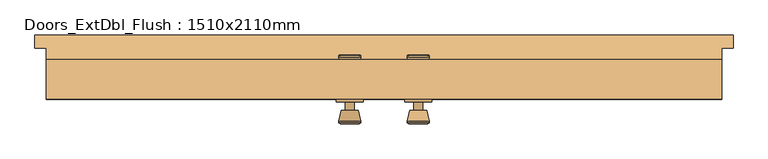
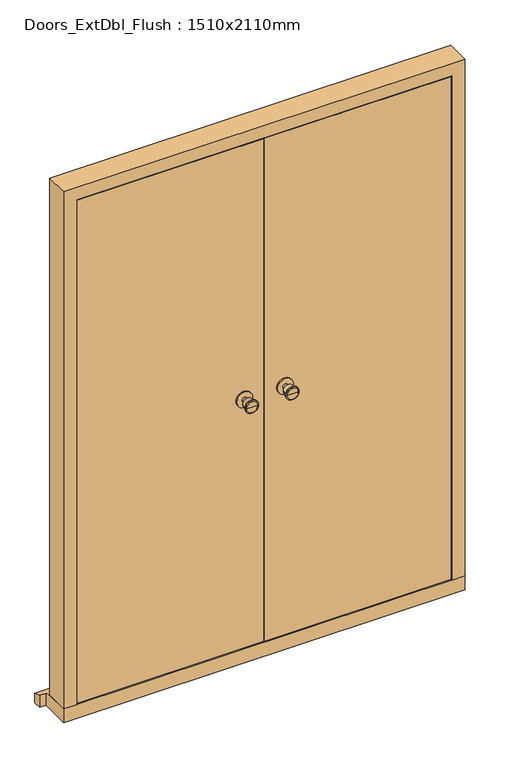
"""IFC4 building model written with IfcOpenShell, lengths in millimetres: door geometry, Doors_ExtDbl_Flush : 1510x2110mm."""

from ifc_helpers import new_model, si_unit, point, frame, frame_2d, origin, place, context, project, spatial, polyline, circle_curve, trimmed, segment, composite_curve, outline, extrude, faceted_brep, source, transform, mapped, element, save
from ifc_brep_helpers import plane_surface, cylinder_surface, revolved_surface, advanced_brep


def doors_extdbl_flush_1510x2110mm_6aadbff8(model_context):
    return source(origin(), model_context, "Body", "SolidModel", [
        advanced_brep(
        [(-76.5, -62.85, 1050.0), (-66.5, -62.85, 1050.0), (-86.5, -62.85, 1050.0), (-96.9758676, -111.85, 1050.0), (-56.0241324, -111.85, 1050.0), (-76.5, -111.85, 1050.0), (-101.5, -110.0221319, 1050.0), (-51.5, -110.0221319, 1050.0), (-101.5, -106.5584537, 1050.0), (-51.5, -106.5584537, 1050.0), (-95.136236, -81.85, 1050.0), (-57.863764, -81.85, 1050.0), (-86.5, -81.85, 1050.0), (-66.5, -81.85, 1050.0)],
        [
            (0, 1),
            (1, 2, circle_curve(frame((-76.5, -62.85, 1050.0), z_axis=(0.0, 1.0, 0.0), x_axis=(1.0, 0.0, 0.0)), 10.0)),
            (2, 0),
            (2, 1, circle_curve(frame((-76.5, -62.85, 1050.0), z_axis=(0.0, 1.0, 0.0), x_axis=(1.0, 0.0, 0.0)), 10.0)),
            (3, 4, circle_curve(frame((-76.5, -111.85, 1050.0), z_axis=(0.0, -1.0, 0.0), x_axis=(1.0, 0.0, 0.0)), 20.4758676)),
            (4, 5),
            (5, 3),
            (4, 3, circle_curve(frame((-76.5, -111.85, 1050.0), z_axis=(0.0, -1.0, 0.0), x_axis=(1.0, 0.0, 0.0)), 20.4758676)),
            (6, 7, circle_curve(frame((-76.5, -110.0221319, 1050.0), z_axis=(0.0, -1.0, 0.0), x_axis=(1.0, 0.0, 0.0)), 25.0)),
            (7, 4),
            (3, 6),
            (7, 6, circle_curve(frame((-76.5, -110.0221319, 1050.0), z_axis=(0.0, -1.0, 0.0), x_axis=(1.0, 0.0, 0.0)), 25.0)),
            (8, 9, circle_curve(frame((-76.5, -106.5584537, 1050.0), z_axis=(0.0, -1.0, 0.0), x_axis=(1.0, 0.0, 0.0)), 25.0)),
            (9, 7),
            (6, 8),
            (9, 8, circle_curve(frame((-76.5, -106.5584537, 1050.0), z_axis=(0.0, -1.0, 0.0), x_axis=(1.0, 0.0, 0.0)), 25.0)),
            (10, 11, circle_curve(frame((-76.5, -81.85, 1050.0), z_axis=(0.0, -1.0, 0.0), x_axis=(1.0, 0.0, 0.0)), 18.636236)),
            (11, 9),
            (8, 10),
            (11, 10, circle_curve(frame((-76.5, -81.85, 1050.0), z_axis=(0.0, -1.0, 0.0), x_axis=(1.0, 0.0, 0.0)), 18.636236)),
            (12, 13, circle_curve(frame((-76.5, -81.85, 1050.0), z_axis=(0.0, -1.0, 0.0), x_axis=(1.0, 0.0, 0.0)), 10.0)),
            (13, 11),
            (10, 12),
            (13, 12, circle_curve(frame((-76.5, -81.85, 1050.0), z_axis=(0.0, -1.0, 0.0), x_axis=(1.0, 0.0, 0.0)), 10.0)),
            (1, 13),
            (12, 2),
        ],
        [
            plane_surface(frame((-76.5, -62.85, 1050.0), z_axis=(0.0, 1.0, 0.0), x_axis=(1.0, 0.0, 0.0))),
            plane_surface(frame((-76.5, -111.85, 1050.0), z_axis=(0.0, -1.0, 0.0), x_axis=(1.0, 0.0, 0.0))),
            revolved_surface(polyline([(-56.0241324, -111.85, 1050.0), (-51.5, -110.0221319, 1050.0)]), (-76.5, -62.85, 1050.0), (0.0, 1.0, 0.0)),
            cylinder_surface(frame((-76.5, -62.85, 1050.0), z_axis=(0.0, 1.0, 0.0), x_axis=(1.0, 0.0, 0.0)), 25.0),
            revolved_surface(polyline([(-51.5, -106.5584537, 1050.0), (-57.863764, -81.85, 1050.0)]), (-76.5, -62.85, 1050.0), (0.0, 1.0, 0.0)),
            plane_surface(frame((-76.5, -81.85, 1050.0), z_axis=(0.0, 1.0, 0.0), x_axis=(1.0, 0.0, 0.0))),
            cylinder_surface(frame((-76.5, -62.85, 1050.0), z_axis=(0.0, 1.0, 0.0), x_axis=(1.0, 0.0, 0.0)), 10.0),
        ],
        [
            (0, [[1, 2, 3]]),
            (0, [[-3, 4, -1]]),
            (1, [[5, 6, 7]]),
            (1, [[8, -7, -6]]),
            (2, [[9, 10, -5, 11]]),
            (2, [[12, -11, -8, -10]]),
            (3, [[13, 14, -9, 15]]),
            (3, [[16, -15, -12, -14]]),
            (4, [[17, 18, -13, 19]]),
            (4, [[20, -19, -16, -18]]),
            (5, [[21, 22, -17, 23]]),
            (5, [[24, -23, -20, -22]]),
            (6, [[-2, 25, -21, 26]]),
            (6, [[-4, -26, -24, -25]]),
        ],
    ),
        extrude(outline(composite_curve([segment(trimmed(circle_curve(frame_2d((1050.0, -76.5)), 30.0), [point((1050.0, -46.5))], [point((1050.0, -106.5))], False, "CARTESIAN"), True, "CONTINUOUS"), segment(trimmed(circle_curve(frame_2d((1050.0, -76.5)), 30.0), [point((1050.0, -106.5))], [point((1050.0, -46.5))], False, "CARTESIAN"), True, "CONTINUOUS")], self_intersect=False)), frame((0.0, -62.85, 0.0), z_axis=(0.0, 1.0, 0.0), x_axis=(0.0, 0.0, 1.0)), (0.0, 0.0, 1.0), 6.0),
        advanced_brep(
        [(-76.5, -6.85, 1050.0), (-86.5, -6.85, 1050.0), (-66.5, -6.85, 1050.0), (-96.9758676, 42.15, 1050.0), (-76.5, 42.15, 1050.0), (-56.0241324, 42.15, 1050.0), (-101.5, 40.3221319, 1050.0), (-51.5, 40.3221319, 1050.0), (-101.5, 36.8584537, 1050.0), (-51.5, 36.8584537, 1050.0), (-95.136236, 12.15, 1050.0), (-57.863764, 12.15, 1050.0), (-86.5, 12.15, 1050.0), (-66.5, 12.15, 1050.0)],
        [
            (0, 1),
            (1, 2, circle_curve(frame((-76.5, -6.85, 1050.0), z_axis=(0.0, -1.0, 0.0), x_axis=(1.0, 0.0, 0.0)), 10.0)),
            (2, 0),
            (2, 1, circle_curve(frame((-76.5, -6.85, 1050.0), z_axis=(0.0, -1.0, 0.0), x_axis=(1.0, 0.0, 0.0)), 10.0)),
            (3, 4),
            (4, 5),
            (5, 3, circle_curve(frame((-76.5, 42.15, 1050.0), z_axis=(0.0, 1.0, 0.0), x_axis=(1.0, 0.0, 0.0)), 20.4758676)),
            (3, 5, circle_curve(frame((-76.5, 42.15, 1050.0), z_axis=(0.0, 1.0, 0.0), x_axis=(1.0, 0.0, 0.0)), 20.4758676)),
            (6, 3),
            (5, 7),
            (7, 6, circle_curve(frame((-76.5, 40.3221319, 1050.0), z_axis=(0.0, 1.0, 0.0), x_axis=(1.0, 0.0, 0.0)), 25.0)),
            (6, 7, circle_curve(frame((-76.5, 40.3221319, 1050.0), z_axis=(0.0, 1.0, 0.0), x_axis=(1.0, 0.0, 0.0)), 25.0)),
            (8, 6),
            (7, 9),
            (9, 8, circle_curve(frame((-76.5, 36.8584537, 1050.0), z_axis=(0.0, 1.0, 0.0), x_axis=(1.0, 0.0, 0.0)), 25.0)),
            (8, 9, circle_curve(frame((-76.5, 36.8584537, 1050.0), z_axis=(0.0, 1.0, 0.0), x_axis=(1.0, 0.0, 0.0)), 25.0)),
            (10, 8),
            (9, 11),
            (11, 10, circle_curve(frame((-76.5, 12.15, 1050.0), z_axis=(0.0, 1.0, 0.0), x_axis=(1.0, 0.0, 0.0)), 18.636236)),
            (10, 11, circle_curve(frame((-76.5, 12.15, 1050.0), z_axis=(0.0, 1.0, 0.0), x_axis=(1.0, 0.0, 0.0)), 18.636236)),
            (12, 10),
            (11, 13),
            (13, 12, circle_curve(frame((-76.5, 12.15, 1050.0), z_axis=(0.0, 1.0, 0.0), x_axis=(1.0, 0.0, 0.0)), 10.0)),
            (12, 13, circle_curve(frame((-76.5, 12.15, 1050.0), z_axis=(0.0, 1.0, 0.0), x_axis=(1.0, 0.0, 0.0)), 10.0)),
            (1, 12),
            (13, 2),
        ],
        [
            plane_surface(frame((-76.5, -6.85, 1050.0), z_axis=(0.0, -1.0, 0.0), x_axis=(1.0, 0.0, 0.0))),
            plane_surface(frame((-76.5, 42.15, 1050.0), z_axis=(0.0, 1.0, 0.0), x_axis=(1.0, 0.0, 0.0))),
            revolved_surface(polyline([(-56.0241324, 42.15, 1050.0), (-51.5, 40.3221319, 1050.0)]), (-76.5, -6.85, 1050.0), (0.0, -1.0, 0.0)),
            cylinder_surface(frame((-76.5, -6.85, 1050.0), z_axis=(0.0, -1.0, 0.0), x_axis=(1.0, 0.0, 0.0)), 25.0),
            revolved_surface(polyline([(-51.5, 36.8584537, 1050.0), (-57.863764, 12.15, 1050.0)]), (-76.5, -6.85, 1050.0), (0.0, -1.0, 0.0)),
            plane_surface(frame((-76.5, 12.15, 1050.0), z_axis=(0.0, -1.0, 0.0), x_axis=(1.0, 0.0, 0.0))),
            cylinder_surface(frame((-76.5, -6.85, 1050.0), z_axis=(0.0, -1.0, 0.0), x_axis=(1.0, 0.0, 0.0)), 10.0),
        ],
        [
            (0, [[1, 2, 3]]),
            (0, [[-3, 4, -1]]),
            (1, [[5, 6, 7]]),
            (1, [[-6, -5, 8]]),
            (2, [[9, -7, 10, 11]]),
            (2, [[-10, -8, -9, 12]]),
            (3, [[13, -11, 14, 15]]),
            (3, [[-14, -12, -13, 16]]),
            (4, [[17, -15, 18, 19]]),
            (4, [[-18, -16, -17, 20]]),
            (5, [[21, -19, 22, 23]]),
            (5, [[-22, -20, -21, 24]]),
            (6, [[25, -23, 26, -2]]),
            (6, [[-26, -24, -25, -4]]),
        ],
    ),
        extrude(outline(composite_curve([segment(trimmed(circle_curve(frame_2d((1050.0, -76.5)), 30.0), [point((1050.0, -46.5))], [point((1050.0, -106.5))], False, "CARTESIAN"), True, "CONTINUOUS"), segment(trimmed(circle_curve(frame_2d((1050.0, -76.5)), 30.0), [point((1050.0, -106.5))], [point((1050.0, -46.5))], False, "CARTESIAN"), True, "CONTINUOUS")], self_intersect=False)), frame((0.0, -12.85, 0.0), z_axis=(0.0, 1.0, 0.0), x_axis=(0.0, 0.0, 1.0)), (0.0, 0.0, 1.0), 6.0),
        advanced_brep(
        [(76.5, -62.85, 1050.0), (86.5, -62.85, 1050.0), (66.5, -62.85, 1050.0), (96.9758676, -111.85, 1050.0), (76.5, -111.85, 1050.0), (56.0241324, -111.85, 1050.0), (101.5, -110.0221319, 1050.0), (51.5, -110.0221319, 1050.0), (101.5, -106.5584537, 1050.0), (51.5, -106.5584537, 1050.0), (95.136236, -81.85, 1050.0), (57.863764, -81.85, 1050.0), (86.5, -81.85, 1050.0), (66.5, -81.85, 1050.0)],
        [
            (0, 1),
            (1, 2, circle_curve(frame((76.5, -62.85, 1050.0), z_axis=(0.0, 1.0, 0.0), x_axis=(-1.0, 0.0, 0.0)), 10.0)),
            (2, 0),
            (2, 1, circle_curve(frame((76.5, -62.85, 1050.0), z_axis=(0.0, 1.0, 0.0), x_axis=(-1.0, 0.0, 0.0)), 10.0)),
            (3, 4),
            (4, 5),
            (5, 3, circle_curve(frame((76.5, -111.85, 1050.0), z_axis=(0.0, -1.0, 0.0), x_axis=(-1.0, 0.0, 0.0)), 20.4758676)),
            (3, 5, circle_curve(frame((76.5, -111.85, 1050.0), z_axis=(0.0, -1.0, 0.0), x_axis=(-1.0, 0.0, 0.0)), 20.4758676)),
            (6, 3),
            (5, 7),
            (7, 6, circle_curve(frame((76.5, -110.0221319, 1050.0), z_axis=(0.0, -1.0, 0.0), x_axis=(-1.0, 0.0, 0.0)), 25.0)),
            (6, 7, circle_curve(frame((76.5, -110.0221319, 1050.0), z_axis=(0.0, -1.0, 0.0), x_axis=(-1.0, 0.0, 0.0)), 25.0)),
            (8, 6),
            (7, 9),
            (9, 8, circle_curve(frame((76.5, -106.5584537, 1050.0), z_axis=(0.0, -1.0, 0.0), x_axis=(-1.0, 0.0, 0.0)), 25.0)),
            (8, 9, circle_curve(frame((76.5, -106.5584537, 1050.0), z_axis=(0.0, -1.0, 0.0), x_axis=(-1.0, 0.0, 0.0)), 25.0)),
            (10, 8),
            (9, 11),
            (11, 10, circle_curve(frame((76.5, -81.85, 1050.0), z_axis=(0.0, -1.0, 0.0), x_axis=(-1.0, 0.0, 0.0)), 18.636236)),
            (10, 11, circle_curve(frame((76.5, -81.85, 1050.0), z_axis=(0.0, -1.0, 0.0), x_axis=(-1.0, 0.0, 0.0)), 18.636236)),
            (12, 10),
            (11, 13),
            (13, 12, circle_curve(frame((76.5, -81.85, 1050.0), z_axis=(0.0, -1.0, 0.0), x_axis=(-1.0, 0.0, 0.0)), 10.0)),
            (12, 13, circle_curve(frame((76.5, -81.85, 1050.0), z_axis=(0.0, -1.0, 0.0), x_axis=(-1.0, 0.0, 0.0)), 10.0)),
            (1, 12),
            (13, 2),
        ],
        [
            plane_surface(frame((76.5, -62.85, 1050.0), z_axis=(0.0, 1.0, 0.0), x_axis=(-1.0, 0.0, 0.0))),
            plane_surface(frame((76.5, -111.85, 1050.0), z_axis=(0.0, -1.0, 0.0), x_axis=(-1.0, 0.0, 0.0))),
            revolved_surface(polyline([(56.0241324, -111.85, 1050.0), (51.5, -110.0221319, 1050.0)]), (76.5, -62.85, 1050.0), (0.0, 1.0, 0.0)),
            cylinder_surface(frame((76.5, -62.85, 1050.0), z_axis=(0.0, 1.0, 0.0), x_axis=(-1.0, 0.0, 0.0)), 25.0),
            revolved_surface(polyline([(51.5, -106.5584537, 1050.0), (57.863764, -81.85, 1050.0)]), (76.5, -62.85, 1050.0), (0.0, 1.0, 0.0)),
            plane_surface(frame((76.5, -81.85, 1050.0), z_axis=(0.0, 1.0, 0.0), x_axis=(-1.0, 0.0, 0.0))),
            cylinder_surface(frame((76.5, -62.85, 1050.0), z_axis=(0.0, 1.0, 0.0), x_axis=(-1.0, 0.0, 0.0)), 10.0),
        ],
        [
            (0, [[1, 2, 3]]),
            (0, [[-3, 4, -1]]),
            (1, [[5, 6, 7]]),
            (1, [[-6, -5, 8]]),
            (2, [[9, -7, 10, 11]]),
            (2, [[-10, -8, -9, 12]]),
            (3, [[13, -11, 14, 15]]),
            (3, [[-14, -12, -13, 16]]),
            (4, [[17, -15, 18, 19]]),
            (4, [[-18, -16, -17, 20]]),
            (5, [[21, -19, 22, 23]]),
            (5, [[-22, -20, -21, 24]]),
            (6, [[25, -23, 26, -2]]),
            (6, [[-26, -24, -25, -4]]),
        ],
    ),
        extrude(outline(composite_curve([segment(trimmed(circle_curve(frame_2d((1050.0, 76.5)), 30.0), [point((1050.0, 46.5))], [point((1050.0, 106.5))], False, "CARTESIAN"), True, "CONTINUOUS"), segment(trimmed(circle_curve(frame_2d((1050.0, 76.5)), 30.0), [point((1050.0, 106.5))], [point((1050.0, 46.5))], False, "CARTESIAN"), True, "CONTINUOUS")], self_intersect=False)), frame((0.0, -62.85, 0.0), z_axis=(0.0, 1.0, 0.0), x_axis=(0.0, 0.0, 1.0)), (0.0, 0.0, 1.0), 6.0),
        advanced_brep(
        [(76.5, -6.85, 1050.0), (66.5, -6.85, 1050.0), (86.5, -6.85, 1050.0), (96.9758676, 42.15, 1050.0), (56.0241324, 42.15, 1050.0), (76.5, 42.15, 1050.0), (101.5, 40.3221319, 1050.0), (51.5, 40.3221319, 1050.0), (101.5, 36.8584537, 1050.0), (51.5, 36.8584537, 1050.0), (95.136236, 12.15, 1050.0), (57.863764, 12.15, 1050.0), (86.5, 12.15, 1050.0), (66.5, 12.15, 1050.0)],
        [
            (0, 1),
            (1, 2, circle_curve(frame((76.5, -6.85, 1050.0), z_axis=(0.0, -1.0, 0.0), x_axis=(-1.0, 0.0, 0.0)), 10.0)),
            (2, 0),
            (2, 1, circle_curve(frame((76.5, -6.85, 1050.0), z_axis=(0.0, -1.0, 0.0), x_axis=(-1.0, 0.0, 0.0)), 10.0)),
            (3, 4, circle_curve(frame((76.5, 42.15, 1050.0), z_axis=(0.0, 1.0, 0.0), x_axis=(-1.0, 0.0, 0.0)), 20.4758676)),
            (4, 5),
            (5, 3),
            (4, 3, circle_curve(frame((76.5, 42.15, 1050.0), z_axis=(0.0, 1.0, 0.0), x_axis=(-1.0, 0.0, 0.0)), 20.4758676)),
            (6, 7, circle_curve(frame((76.5, 40.3221319, 1050.0), z_axis=(0.0, 1.0, 0.0), x_axis=(-1.0, 0.0, 0.0)), 25.0)),
            (7, 4),
            (3, 6),
            (7, 6, circle_curve(frame((76.5, 40.3221319, 1050.0), z_axis=(0.0, 1.0, 0.0), x_axis=(-1.0, 0.0, 0.0)), 25.0)),
            (8, 9, circle_curve(frame((76.5, 36.8584537, 1050.0), z_axis=(0.0, 1.0, 0.0), x_axis=(-1.0, 0.0, 0.0)), 25.0)),
            (9, 7),
            (6, 8),
            (9, 8, circle_curve(frame((76.5, 36.8584537, 1050.0), z_axis=(0.0, 1.0, 0.0), x_axis=(-1.0, 0.0, 0.0)), 25.0)),
            (10, 11, circle_curve(frame((76.5, 12.15, 1050.0), z_axis=(0.0, 1.0, 0.0), x_axis=(-1.0, 0.0, 0.0)), 18.636236)),
            (11, 9),
            (8, 10),
            (11, 10, circle_curve(frame((76.5, 12.15, 1050.0), z_axis=(0.0, 1.0, 0.0), x_axis=(-1.0, 0.0, 0.0)), 18.636236)),
            (12, 13, circle_curve(frame((76.5, 12.15, 1050.0), z_axis=(0.0, 1.0, 0.0), x_axis=(-1.0, 0.0, 0.0)), 10.0)),
            (13, 11),
            (10, 12),
            (13, 12, circle_curve(frame((76.5, 12.15, 1050.0), z_axis=(0.0, 1.0, 0.0), x_axis=(-1.0, 0.0, 0.0)), 10.0)),
            (1, 13),
            (12, 2),
        ],
        [
            plane_surface(frame((76.5, -6.85, 1050.0), z_axis=(0.0, -1.0, 0.0), x_axis=(-1.0, 0.0, 0.0))),
            plane_surface(frame((76.5, 42.15, 1050.0), z_axis=(0.0, 1.0, 0.0), x_axis=(-1.0, 0.0, 0.0))),
            revolved_surface(polyline([(56.0241324, 42.15, 1050.0), (51.5, 40.3221319, 1050.0)]), (76.5, -6.85, 1050.0), (0.0, -1.0, 0.0)),
            cylinder_surface(frame((76.5, -6.85, 1050.0), z_axis=(0.0, -1.0, 0.0), x_axis=(-1.0, 0.0, 0.0)), 25.0),
            revolved_surface(polyline([(51.5, 36.8584537, 1050.0), (57.863764, 12.15, 1050.0)]), (76.5, -6.85, 1050.0), (0.0, -1.0, 0.0)),
            plane_surface(frame((76.5, 12.15, 1050.0), z_axis=(0.0, -1.0, 0.0), x_axis=(-1.0, 0.0, 0.0))),
            cylinder_surface(frame((76.5, -6.85, 1050.0), z_axis=(0.0, -1.0, 0.0), x_axis=(-1.0, 0.0, 0.0)), 10.0),
        ],
        [
            (0, [[1, 2, 3]]),
            (0, [[-3, 4, -1]]),
            (1, [[5, 6, 7]]),
            (1, [[8, -7, -6]]),
            (2, [[9, 10, -5, 11]]),
            (2, [[12, -11, -8, -10]]),
            (3, [[13, 14, -9, 15]]),
            (3, [[16, -15, -12, -14]]),
            (4, [[17, 18, -13, 19]]),
            (4, [[20, -19, -16, -18]]),
            (5, [[21, 22, -17, 23]]),
            (5, [[24, -23, -20, -22]]),
            (6, [[-2, 25, -21, 26]]),
            (6, [[-4, -26, -24, -25]]),
        ],
    ),
        extrude(outline(composite_curve([segment(trimmed(circle_curve(frame_2d((1050.0, 76.5)), 30.0), [point((1050.0, 46.5))], [point((1050.0, 106.5))], False, "CARTESIAN"), True, "CONTINUOUS"), segment(trimmed(circle_curve(frame_2d((1050.0, 76.5)), 30.0), [point((1050.0, 106.5))], [point((1050.0, 46.5))], False, "CARTESIAN"), True, "CONTINUOUS")], self_intersect=False)), frame((0.0, -12.85, 0.0), z_axis=(0.0, 1.0, 0.0), x_axis=(0.0, 0.0, 1.0)), (0.0, 0.0, 1.0), 6.0),
        faceted_brep([(684.5, 32.15, 54.5), (755.0, 32.15, 54.5), (755.0, -56.85, 54.5), (706.5, -56.85, 54.5), (706.5, -9.85, 54.5), (684.5, -9.85, 54.5), (684.5, 32.15, 2039.5), (-684.5, 32.15, 2039.5), (-684.5, 32.15, 54.5), (-755.0, 32.15, 54.5), (-755.0, 32.15, 2110.0), (755.0, 32.15, 2110.0), (755.0, -56.85, 2110.0), (-755.0, -56.85, 2110.0), (-755.0, -56.85, 54.5), (-706.5, -56.85, 54.5), (-706.5, -56.85, 2061.5), (706.5, -56.85, 2061.5), (706.5, -9.85, 2061.5), (-706.5, -9.85, 2061.5), (-706.5, -9.85, 54.5), (-684.5, -9.85, 54.5), (-684.5, -9.85, 2039.5), (684.5, -9.85, 2039.5)], [[[0, 1, 2, 3, 4, 5]], [[1, 0, 6, 7, 8, 9, 10, 11]], [[2, 1, 11, 12]], [[3, 2, 12, 13, 14, 15, 16, 17]], [[4, 3, 17, 18]], [[5, 4, 18, 19, 20, 21, 22, 23]], [[0, 5, 23, 6]], [[12, 11, 10, 13]], [[18, 17, 16, 19]], [[6, 23, 22, 7]], [[8, 21, 20, 15, 14, 9]], [[13, 10, 9, 14]], [[19, 16, 15, 20]], [[7, 22, 21, 8]]]),
        faceted_brep([(780.0, 87.15, 0.0), (780.0, 87.15, 38.5947221), (780.0, 57.15, 47.2703282), (780.0, 57.15, 0.0), (-780.0, 87.15, 38.5947221), (-780.0, 87.15, 0.0), (-780.0, 57.15, 0.0), (-780.0, 57.15, 47.2703282), (755.0, 57.15, 0.0), (755.0, -56.85, 0.0), (-755.0, -56.85, 0.0), (-755.0, 57.15, 0.0), (-755.0, 57.15, 47.2703282), (-755.0, 32.15, 54.5), (755.0, 32.15, 54.5), (755.0, 57.15, 47.2703282), (-755.0, -56.85, 54.5), (755.0, -56.85, 54.5)], [[[0, 1, 2, 3]], [[4, 5, 6, 7]], [[5, 0, 3, 8, 9, 10, 11, 6]], [[1, 0, 5, 4]], [[1, 4, 7, 12, 13, 14, 15, 2]], [[13, 16, 17, 14]], [[16, 10, 9, 17]], [[12, 11, 10, 16, 13]], [[11, 12, 7, 6]], [[8, 15, 14, 17, 9]], [[15, 8, 3, 2]]]),
        extrude(outline(polyline([(703.5, -56.85), (1.5, -56.85), (1.5, -12.85), (703.5, -12.85), (703.5, -56.85)])), frame((0.0, 0.0, 58.5), z_axis=(0.0, 0.0, 1.0), x_axis=(1.0, 0.0, 0.0)), (0.0, 0.0, 1.0), 2000.0),
        extrude(outline(polyline([(-1.5, -56.85), (-703.5, -56.85), (-703.5, -12.85), (-1.5, -12.85), (-1.5, -56.85)])), frame((0.0, 0.0, 58.5), z_axis=(0.0, 0.0, 1.0), x_axis=(1.0, 0.0, 0.0)), (0.0, 0.0, 1.0), 2000.0),
    ])


if __name__ == "__main__":
    model = new_model("IFC4")
    model_context = context("Model", 3, world=origin())
    ifc_project = project(units=[si_unit("LENGTHUNIT", "METRE", prefix="MILLI")], contexts=[model_context])
    site = spatial("IfcSite", under=ifc_project)
    building = spatial("IfcBuilding", under=site)
    placement = place(None, origin())
    doors_extdbl_flush_1510x2110mm_shape = doors_extdbl_flush_1510x2110mm_6aadbff8(model_context)
    element("IfcDoor", 1, ObjectType="Doors_ExtDbl_Flush : 1510x2110mm", at=placement, inside=building, context=model_context, shape_type="MappedRepresentation", body=[
        mapped(doors_extdbl_flush_1510x2110mm_shape, transform((0.0, 0.0, 0.0), x_axis=(1.0, 0.0, 0.0), y_axis=(0.0, 1.0, 0.0), z_axis=(0.0, 0.0, 1.0))),
    ])
    save(model, "model.ifc")

# Revit data of these elements
# Type "Doors_ExtDbl_Flush : 1510x2110mm"
#   Construction Type Id = "MDOOR"
#   Type Mark = "45"
#   Type Comments = "External Double"
#   Operation = "DoubleDoorSingleSwing"
#   Keynote = "L20"
#   Analytic Construction = "Metal"
#   Wrap Layers (Ext) from Ext = 0' - 4.03543"
#   Wrap Layers (Int) from Ext = 0' - 6.98819"
#   Thickness = 0' - 1.73228"
#   Rough Width = 4' - 11.44882"
#   Rough Height = 6' - 11.07087"
#   O/A Frame Width = 0' - 2.51969"
#   Heat Transfer Coefficient (U) = 3.7021 W/(m²·K)
#   Handle Z Distance = 3' - 5.33858"
#   FrameWidth = 0' - 1.65354"
#   FrameOffset - External = 0' - 0.98425"
#   FrameDepth = 0' - 3.50394"
#   Door Panel Width = 2' - 3.6378"
#   Door Panel Thickness = 0' - 1.73228"
#   Door Panel Height = 6' - 6.74016"
#   Cill Thickness = 0' - 2.14567"
#   Cill Projection = 0' - 1.1811"
#   Handle X Distance = 0' - 2.95276"
#   Height = 6' - 11.07087"
#   Structural Tolerance = 0' - 0.25591"
#   Tolerance = 0' - 0.11811"
#   Undercut = 0' - 0.15748"
#   Width = 4' - 11.44882"
#   Cill Extension = 0' - 0.98425"
#   Cavity Closer Width = 0' - 1.9685"
#   Cavity Closer Offset from Ext = 0' - 4.03543"
#   Cavity Closer Depth = 0' - 3.34646"
#   Define Thermal Properties by = 1
#   Vis - Ironmongery = yes
#   Vis - Cavity Closers = yes
#   Function = 1
#   Material Door = Door - Panel
#   Material Frame = Door - Frame/Mullion
#   Material Ironmongery = Door - Handle
#   Visual Light Transmittance = 0
#   Thermal Resistance (R) = 0
#   Solar Heat Gain Coefficient = 0
#   Wall Closure = (empty or 0)
# Element 1 (IfcDoor, "Doors_ExtDbl_Flush : 1510x2110mm")
#   Materials on its faces: "Door - Handle", "Door - Frame/Mullion", "Door - Panel"
# Materials
#   "Door - Panel": class "Wood", colour RGB 210 159 95, transparency 0, Keynote = "L20", Cost = 0
#   "Door - Frame/Mullion": class "Wood", colour RGB 212 179 113, transparency 0, Keynote = "L20", Cost = 0
#   "Door - Handle": colour RGB 17 17 17, transparency 0, Keynote = "P21", Cost = 0
